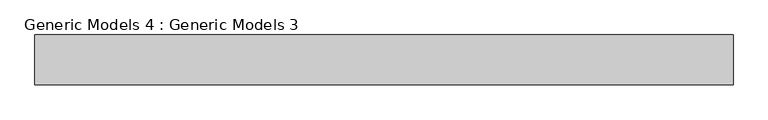
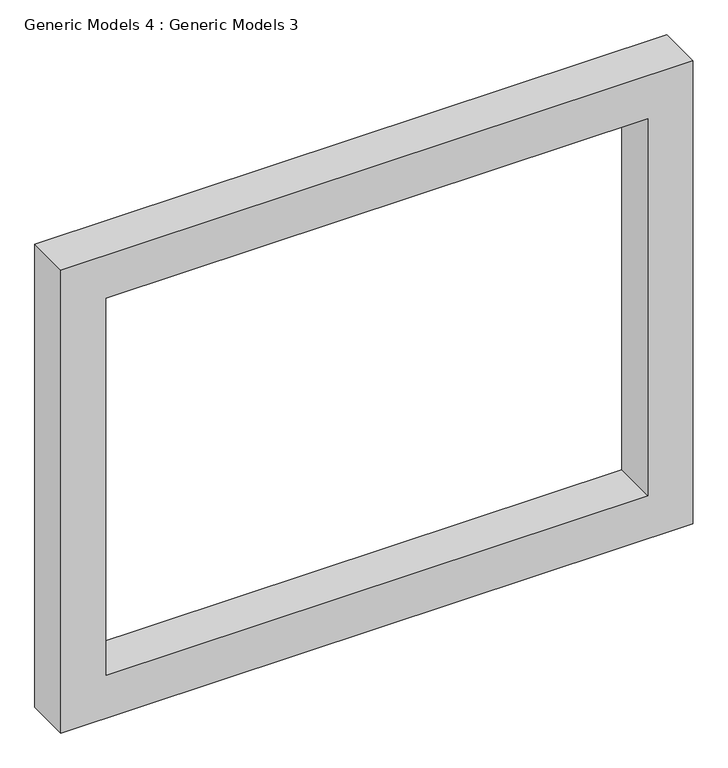
"""IFC4 building model written with IfcOpenShell, lengths in millimetres: proxy geometry, Generic Models 4 : Generic Models 3."""

from ifc_helpers import new_model, si_unit, frame, origin, place, context, project, spatial, polyline, outline, extrude, source, transform, mapped, element, save


def generic_models_4_generic_models_3_cea7143c(model_context):
    return source(origin(), model_context, "Body", "SweptSolid", [
        extrude(outline(polyline([(5765.8, -2072.1328791), (5765.8, -4205.7328791), (4114.8, -4205.7328791), (4114.8, -2072.1328791), (5765.8, -2072.1328791)]), holes=[polyline([(5613.4, -2224.5328791), (4267.2, -2224.5328791), (4267.2, -4053.3328791), (5613.4, -4053.3328791), (5613.4, -2224.5328791)])]), frame((0.0, -2602.2776789, 0.0), z_axis=(0.0, 1.0, 0.0), x_axis=(0.0, 0.0, 1.0)), (0.0, 0.0, 1.0), 152.4),
    ])


if __name__ == "__main__":
    model = new_model("IFC4")
    model_context = context("Model", 3, world=origin())
    ifc_project = project(units=[si_unit("LENGTHUNIT", "METRE", prefix="MILLI")], contexts=[model_context])
    site = spatial("IfcSite", under=ifc_project)
    building = spatial("IfcBuilding", under=site)
    placement = place(None, origin())
    generic_models_4_generic_models_3_shape = generic_models_4_generic_models_3_cea7143c(model_context)
    element("IfcBuildingElementProxy", 1, Name="Generic Models 4 : Generic Models 3", ObjectType="Generic Models 4 : Generic Models 3", at=placement, inside=building, context=model_context, shape_type="MappedRepresentation", body=[
        mapped(generic_models_4_generic_models_3_shape, transform((0.0, 0.0, 0.0), x_axis=(1.0, 0.0, 0.0), y_axis=(0.0, 1.0, 0.0), z_axis=(0.0, 0.0, 1.0))),
    ])
    save(model, "model.ifc")

# Revit data of these elements
# Element 1 (IfcBuildingElementProxy, "Generic Models 4 : Generic Models 3")
#   Materials on its faces: "WALNUT WOOD COLOUR 5\""
# Materials
#   "WALNUT WOOD COLOUR 5\"": class "Generic", colour RGB 120 120 120, transparency 0, Cost = 0
